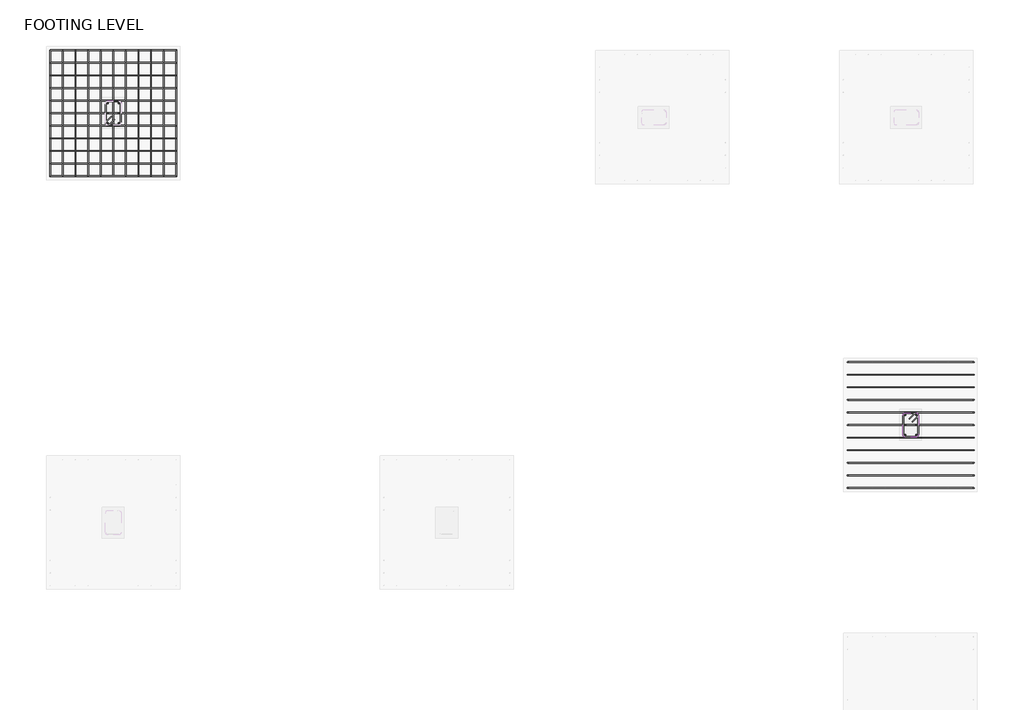
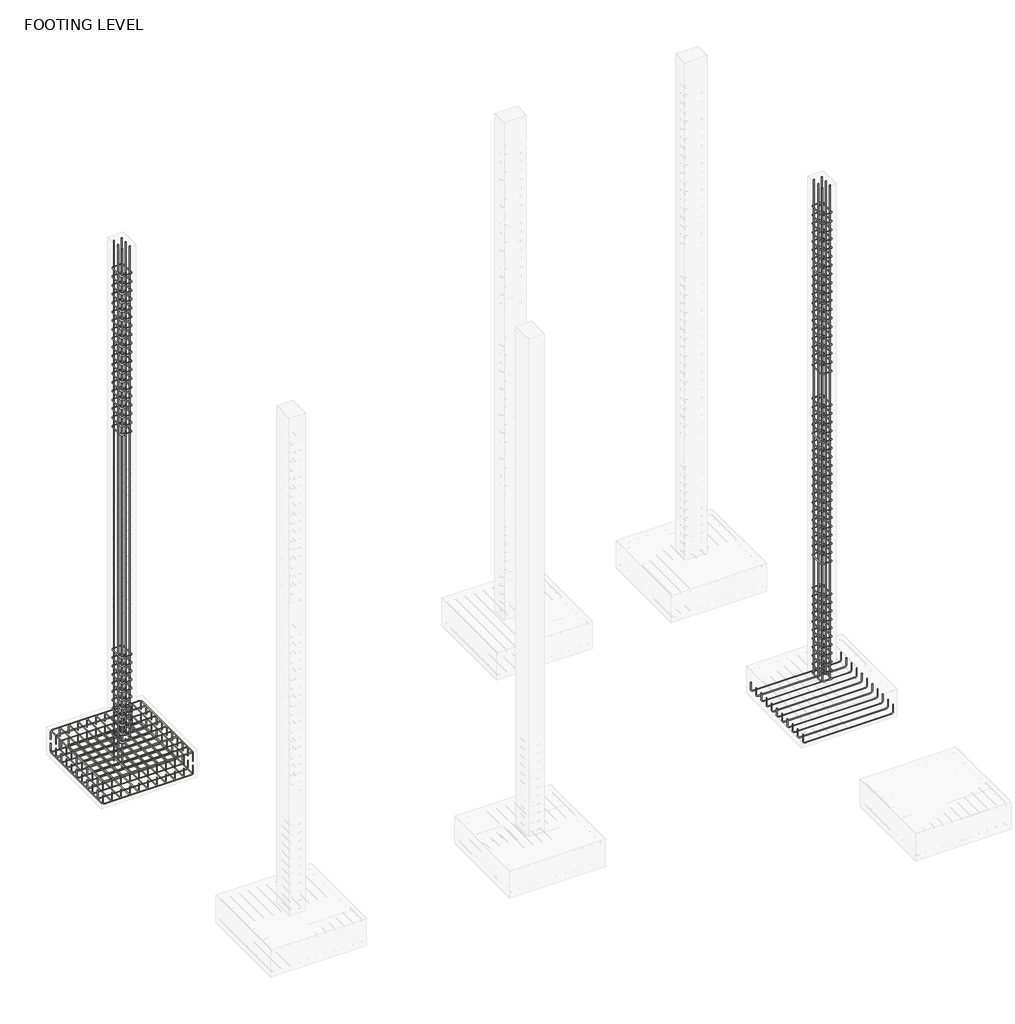
# One storey, part 6 of 9: 22 reinforcing bars.
"""IFC4 building model written with IfcOpenShell, lengths in millimetres."""

from ifc_helpers import new_model, si_unit, point, frame, origin, place, context, project, spatial, polyline, circle_curve, trimmed, segment, composite_curve, source, transform, mapped, element, save
from ifc_brep_helpers import swept_disk

model = new_model("IFC4")

# Units and contexts
model_context = context("Model", 3, world=origin())
ifc_project = project(units=[si_unit("LENGTHUNIT", "METRE", prefix="MILLI")], contexts=[model_context])

# Site, building, storey
site = spatial("IfcSite", under=ifc_project)
building = spatial("IfcBuilding", under=site)
storey = spatial("IfcBuildingStorey", under=building, Name="FOOTING LEVEL", Elevation=-1981.2)

# Reinforcing bars
placement = place(None, origin())
reinforcing_bar_shape = source(origin(), model_context, "Body", "SolidModel", [
    swept_disk(composite_curve([segment(polyline([(-12382.3821491, 8189.9555175, -1938.3375), (-12439.2463461, 8133.0913204, -1938.3375)]), True, "CONTINUOUS"), segment(trimmed(circle_curve(frame((-12422.4083659, 8116.2533402, -1938.3375), z_axis=(0.0, 0.0, 1.0), x_axis=(-16.837980199999947, 16.837980199999947, 0.0)), 23.8125), [point((-12439.2463461, 8133.0913204, -1938.3375))], [point((-12422.4083659, 8092.4408402, -1938.3375))], True, "CARTESIAN"), True, "CONTINUOUS"), segment(polyline([(-12422.4083659, 8092.4408402, -1938.3375), (-12301.7583659, 8092.4408402, -1938.3375)]), True, "CONTINUOUS"), segment(trimmed(circle_curve(frame((-12301.7583659, 8116.2533402, -1938.3375), z_axis=(0.0, 0.0, 1.0), x_axis=(0.0, -23.8125, 0.0)), 23.8125), [point((-12301.7583659, 8092.4408402, -1938.3375))], [point((-12277.9458659, 8116.2533402, -1938.3375))], True, "CARTESIAN"), True, "CONTINUOUS"), segment(polyline([(-12277.9458659, 8116.2533402, -1938.3375), (-12277.9458659, 8338.5033402, -1938.3375)]), True, "CONTINUOUS"), segment(trimmed(circle_curve(frame((-12301.7203098, 8338.5033402, -1939.6832232), z_axis=(-0.056513312022656255, 0.0, 0.9984018457335854), x_axis=(23.774443900001643, 0.0, 1.3457231999998385)), 23.8125), [point((-12277.9458659, 8338.5033402, -1938.3375))], [point((-12301.7203098, 8362.3158402, -1939.6832232))], True, "CARTESIAN"), True, "CONTINUOUS"), segment(polyline([(-12301.7203098, 8362.3158402, -1939.6832232), (-12422.4464219, 8362.3158402, -1946.5167768)]), True, "CONTINUOUS"), segment(trimmed(circle_curve(frame((-12422.4464219, 8338.5033402, -1946.5167768), z_axis=(-0.056513312022656255, 0.0, 0.9984018457335854), x_axis=(0.0, 23.8125, 0.0)), 23.8125), [point((-12422.4464219, 8362.3158402, -1946.5167768))], [point((-12446.2208659, 8338.5033402, -1947.8625))], True, "CARTESIAN"), True, "CONTINUOUS"), segment(polyline([(-12446.2208659, 8338.5033402, -1947.8625), (-12446.2208659, 8116.2533402, -1947.8625)]), True, "CONTINUOUS"), segment(trimmed(circle_curve(frame((-12422.4083659, 8116.2533402, -1947.8625), z_axis=(0.0, 0.0, 1.0), x_axis=(-23.8125, 0.0, 0.0)), 23.8125), [point((-12446.2208659, 8116.2533402, -1947.8625))], [point((-12405.5703857, 8099.41536, -1947.8625))], True, "CARTESIAN"), True, "CONTINUOUS"), segment(polyline([(-12405.5703857, 8099.41536, -1947.8625), (-12348.7061886, 8156.279557, -1947.8625)]), True, "CONTINUOUS")], self_intersect=False), 4.7625),
])
element("IfcReinforcingBar", 1, at=placement, inside=storey, context=model_context, shape_type="MappedRepresentation", body=[
    mapped(reinforcing_bar_shape, transform((0.0, 0.0, 0.0), x_axis=(1.0, 0.0, 0.0), y_axis=(0.0, 1.0, 0.0), z_axis=(0.0, 0.0, 1.0))),
    mapped(reinforcing_bar_shape, transform((0.0, 0.0, 142.5866456), x_axis=(1.0, 0.0, 0.0), y_axis=(0.0, 1.0, 0.0), z_axis=(0.0, 0.0, 1.0))),
    mapped(reinforcing_bar_shape, transform((0.0, 0.0, 285.1732912), x_axis=(1.0, 0.0, 0.0), y_axis=(0.0, 1.0, 0.0), z_axis=(0.0, 0.0, 1.0))),
    mapped(reinforcing_bar_shape, transform((0.0, 0.0, 427.7599369), x_axis=(1.0, 0.0, 0.0), y_axis=(0.0, 1.0, 0.0), z_axis=(0.0, 0.0, 1.0))),
    mapped(reinforcing_bar_shape, transform((0.0, 0.0, 570.3465825), x_axis=(1.0, 0.0, 0.0), y_axis=(0.0, 1.0, 0.0), z_axis=(0.0, 0.0, 1.0))),
    mapped(reinforcing_bar_shape, transform((0.0, 0.0, 712.9332281), x_axis=(1.0, 0.0, 0.0), y_axis=(0.0, 1.0, 0.0), z_axis=(0.0, 0.0, 1.0))),
    mapped(reinforcing_bar_shape, transform((0.0, 0.0, 855.5198737), x_axis=(1.0, 0.0, 0.0), y_axis=(0.0, 1.0, 0.0), z_axis=(0.0, 0.0, 1.0))),
    mapped(reinforcing_bar_shape, transform((0.0, 0.0, 998.1065193), x_axis=(1.0, 0.0, 0.0), y_axis=(0.0, 1.0, 0.0), z_axis=(0.0, 0.0, 1.0))),
    mapped(reinforcing_bar_shape, transform((0.0, 0.0, 1140.6931649), x_axis=(1.0, 0.0, 0.0), y_axis=(0.0, 1.0, 0.0), z_axis=(0.0, 0.0, 1.0))),
    mapped(reinforcing_bar_shape, transform((0.0, 0.0, 1283.2798106), x_axis=(1.0, 0.0, 0.0), y_axis=(0.0, 1.0, 0.0), z_axis=(0.0, 0.0, 1.0))),
    mapped(reinforcing_bar_shape, transform((0.0, 0.0, 1425.8664562), x_axis=(1.0, 0.0, 0.0), y_axis=(0.0, 1.0, 0.0), z_axis=(0.0, 0.0, 1.0))),
])
element("IfcReinforcingBar", 2, at=placement, inside=storey, context=model_context, shape_type="SolidModel", body=[
    swept_disk(composite_curve([segment(polyline([(-12423.8882737, 8340.8596793, -2400.3), (-12423.8882737, 8340.8596793, 6362.7)]), True, "CONTINUOUS")], self_intersect=False), 6.35),
])
element("IfcReinforcingBar", 3, at=placement, inside=storey, context=model_context, shape_type="SolidModel", body=[
    swept_disk(composite_curve([segment(polyline([(-12300.2784581, 8340.8596793, -1943.1), (-12300.2784581, 8340.8596793, 6362.7)]), True, "CONTINUOUS")], self_intersect=False), 6.35),
])
element("IfcReinforcingBar", 4, at=placement, inside=storey, context=model_context, shape_type="SolidModel", body=[
    swept_disk(composite_curve([segment(polyline([(-12423.8882737, 8113.8970011, -2400.3), (-12423.8882737, 8113.8970011, 6362.7)]), True, "CONTINUOUS")], self_intersect=False), 6.35),
])
element("IfcReinforcingBar", 5, at=placement, inside=storey, context=model_context, shape_type="SolidModel", body=[
    swept_disk(composite_curve([segment(polyline([(-12300.2784581, 8113.8970011, -1943.1), (-12300.2784581, 8113.8970011, 6362.7)]), True, "CONTINUOUS")], self_intersect=False), 6.35),
])
element("IfcReinforcingBar", 6, at=placement, inside=storey, context=model_context, shape_type="SolidModel", body=[
    swept_disk(composite_curve([segment(polyline([(-12423.8882737, 8228.1970011, -2400.3), (-12423.8882737, 8228.1970011, 6362.7)]), True, "CONTINUOUS")], self_intersect=False), 6.35),
])
element("IfcReinforcingBar", 7, at=placement, inside=storey, context=model_context, shape_type="SolidModel", body=[
    swept_disk(composite_curve([segment(polyline([(-12300.2784581, 8228.1970011, -1943.1), (-12300.2784581, 8228.1970011, 6362.7)]), True, "CONTINUOUS")], self_intersect=False), 6.35),
])
reinforcing_bar_2_shape = source(origin(), model_context, "Body", "SolidModel", [
    swept_disk(composite_curve([segment(polyline([(-3975.4566189, 3944.9119441, -2247.9), (-3975.4566189, 3944.9119441, -2362.2)]), True, "CONTINUOUS"), segment(trimmed(circle_curve(frame((-3942.1191189, 3944.9119441, -2362.2), z_axis=(0.0, -1.0, 0.0), x_axis=(-33.33750000000009, 0.0, 0.0)), 33.3375), [point((-3975.4566189, 3944.9119441, -2362.2))], [point((-3942.1191189, 3944.9119441, -2395.5375))], True, "CARTESIAN"), True, "CONTINUOUS"), segment(polyline([(-3942.1191189, 3944.9119441, -2395.5375), (-2570.5191189, 3944.9119441, -2395.5375)]), True, "CONTINUOUS"), segment(trimmed(circle_curve(frame((-2570.5191189, 3944.9119441, -2362.2), z_axis=(0.0, -1.0, 0.0), x_axis=(0.0, 0.0, -33.33750000000009)), 33.3375), [point((-2570.5191189, 3944.9119441, -2395.5375))], [point((-2537.1816189, 3944.9119441, -2362.2))], True, "CARTESIAN"), True, "CONTINUOUS"), segment(polyline([(-2537.1816189, 3944.9119441, -2362.2), (-2537.1816189, 3944.9119441, -2247.9)]), True, "CONTINUOUS")], self_intersect=False), 4.7625),
])
element("IfcReinforcingBar", 8, at=placement, inside=storey, context=model_context, shape_type="MappedRepresentation", body=[
    mapped(reinforcing_bar_2_shape, transform((0.0, 0.0, 0.0), x_axis=(1.0, 0.0, 0.0), y_axis=(0.0, 1.0, 0.0), z_axis=(0.0, 0.0, 1.0))),
    mapped(reinforcing_bar_2_shape, transform((0.0, 143.8275, 0.0), x_axis=(1.0, 0.0, 0.0), y_axis=(0.0, 1.0, 0.0), z_axis=(0.0, 0.0, 1.0))),
    mapped(reinforcing_bar_2_shape, transform((0.0, 287.655, 0.0), x_axis=(1.0, 0.0, 0.0), y_axis=(0.0, 1.0, 0.0), z_axis=(0.0, 0.0, 1.0))),
    mapped(reinforcing_bar_2_shape, transform((0.0, 431.4825, 0.0), x_axis=(1.0, 0.0, 0.0), y_axis=(0.0, 1.0, 0.0), z_axis=(0.0, 0.0, 1.0))),
    mapped(reinforcing_bar_2_shape, transform((0.0, 575.31, 0.0), x_axis=(1.0, 0.0, 0.0), y_axis=(0.0, 1.0, 0.0), z_axis=(0.0, 0.0, 1.0))),
    mapped(reinforcing_bar_2_shape, transform((0.0, 719.1375, 0.0), x_axis=(1.0, 0.0, 0.0), y_axis=(0.0, 1.0, 0.0), z_axis=(0.0, 0.0, 1.0))),
    mapped(reinforcing_bar_2_shape, transform((0.0, 862.965, 0.0), x_axis=(1.0, 0.0, 0.0), y_axis=(0.0, 1.0, 0.0), z_axis=(0.0, 0.0, 1.0))),
    mapped(reinforcing_bar_2_shape, transform((0.0, 1006.7925, 0.0), x_axis=(1.0, 0.0, 0.0), y_axis=(0.0, 1.0, 0.0), z_axis=(0.0, 0.0, 1.0))),
    mapped(reinforcing_bar_2_shape, transform((0.0, 1150.62, 0.0), x_axis=(1.0, 0.0, 0.0), y_axis=(0.0, 1.0, 0.0), z_axis=(0.0, 0.0, 1.0))),
    mapped(reinforcing_bar_2_shape, transform((0.0, 1294.4475, 0.0), x_axis=(1.0, 0.0, 0.0), y_axis=(0.0, 1.0, 0.0), z_axis=(0.0, 0.0, 1.0))),
    mapped(reinforcing_bar_2_shape, transform((0.0, 1438.275, 0.0), x_axis=(1.0, 0.0, 0.0), y_axis=(0.0, 1.0, 0.0), z_axis=(0.0, 0.0, 1.0))),
])
reinforcing_bar_3_shape = source(origin(), model_context, "Body", "SolidModel", [
    swept_disk(composite_curve([segment(polyline([(-11642.9458659, 8946.5158402, -2171.7), (-11642.9458659, 8946.5158402, -2057.4)]), True, "CONTINUOUS"), segment(trimmed(circle_curve(frame((-11642.9458659, 8913.1783402, -2057.4), z_axis=(1.0, 0.0, 0.0), x_axis=(0.0, 33.337499999999636, 0.0)), 33.3375), [point((-11642.9458659, 8946.5158402, -2057.4))], [point((-11642.9458659, 8913.1783402, -2024.0625))], True, "CARTESIAN"), True, "CONTINUOUS"), segment(polyline([(-11642.9458659, 8913.1783402, -2024.0625), (-11642.9458659, 7541.5783402, -2024.0625)]), True, "CONTINUOUS"), segment(trimmed(circle_curve(frame((-11642.9458659, 7541.5783402, -2057.4), z_axis=(1.0, 0.0, 0.0), x_axis=(0.0, 0.0, 33.33750000000009)), 33.3375), [point((-11642.9458659, 7541.5783402, -2024.0625))], [point((-11642.9458659, 7508.2408402, -2057.4))], True, "CARTESIAN"), True, "CONTINUOUS"), segment(polyline([(-11642.9458659, 7508.2408402, -2057.4), (-11642.9458659, 7508.2408402, -2171.7)]), True, "CONTINUOUS")], self_intersect=False), 4.7625),
])
element("IfcReinforcingBar", 9, at=placement, inside=storey, context=model_context, shape_type="MappedRepresentation", body=[
    mapped(reinforcing_bar_3_shape, transform((0.0, 0.0, 0.0), x_axis=(1.0, 0.0, 0.0), y_axis=(0.0, 1.0, 0.0), z_axis=(0.0, 0.0, 1.0))),
    mapped(reinforcing_bar_3_shape, transform((-143.8275, 0.0, 0.0), x_axis=(1.0, 0.0, 0.0), y_axis=(0.0, 1.0, 0.0), z_axis=(0.0, 0.0, 1.0))),
    mapped(reinforcing_bar_3_shape, transform((-287.655, 0.0, 0.0), x_axis=(1.0, 0.0, 0.0), y_axis=(0.0, 1.0, 0.0), z_axis=(0.0, 0.0, 1.0))),
    mapped(reinforcing_bar_3_shape, transform((-431.4825, 0.0, 0.0), x_axis=(1.0, 0.0, 0.0), y_axis=(0.0, 1.0, 0.0), z_axis=(0.0, 0.0, 1.0))),
    mapped(reinforcing_bar_3_shape, transform((-575.31, 0.0, 0.0), x_axis=(1.0, 0.0, 0.0), y_axis=(0.0, 1.0, 0.0), z_axis=(0.0, 0.0, 1.0))),
    mapped(reinforcing_bar_3_shape, transform((-719.1375, 0.0, 0.0), x_axis=(1.0, 0.0, 0.0), y_axis=(0.0, 1.0, 0.0), z_axis=(0.0, 0.0, 1.0))),
    mapped(reinforcing_bar_3_shape, transform((-862.965, 0.0, 0.0), x_axis=(1.0, 0.0, 0.0), y_axis=(0.0, 1.0, 0.0), z_axis=(0.0, 0.0, 1.0))),
    mapped(reinforcing_bar_3_shape, transform((-1006.7925, 0.0, 0.0), x_axis=(1.0, 0.0, 0.0), y_axis=(0.0, 1.0, 0.0), z_axis=(0.0, 0.0, 1.0))),
    mapped(reinforcing_bar_3_shape, transform((-1150.62, 0.0, 0.0), x_axis=(1.0, 0.0, 0.0), y_axis=(0.0, 1.0, 0.0), z_axis=(0.0, 0.0, 1.0))),
    mapped(reinforcing_bar_3_shape, transform((-1294.4475, 0.0, 0.0), x_axis=(1.0, 0.0, 0.0), y_axis=(0.0, 1.0, 0.0), z_axis=(0.0, 0.0, 1.0))),
    mapped(reinforcing_bar_3_shape, transform((-1438.275, 0.0, 0.0), x_axis=(1.0, 0.0, 0.0), y_axis=(0.0, 1.0, 0.0), z_axis=(0.0, 0.0, 1.0))),
])
reinforcing_bar_4_shape = source(origin(), model_context, "Body", "SolidModel", [
    swept_disk(composite_curve([segment(polyline([(-11642.9458659, 7508.2408402, -2247.9), (-11642.9458659, 7508.2408402, -2362.2)]), True, "CONTINUOUS"), segment(trimmed(circle_curve(frame((-11642.9458659, 7541.5783402, -2362.2), z_axis=(1.0, 0.0, 0.0), x_axis=(0.0, -33.337499999999636, 0.0)), 33.3375), [point((-11642.9458659, 7508.2408402, -2362.2))], [point((-11642.9458659, 7541.5783402, -2395.5375))], True, "CARTESIAN"), True, "CONTINUOUS"), segment(polyline([(-11642.9458659, 7541.5783402, -2395.5375), (-11642.9458659, 8913.1783402, -2395.5375)]), True, "CONTINUOUS"), segment(trimmed(circle_curve(frame((-11642.9458659, 8913.1783402, -2362.2), z_axis=(1.0, 0.0, 0.0), x_axis=(0.0, 0.0, -33.33750000000009)), 33.3375), [point((-11642.9458659, 8913.1783402, -2395.5375))], [point((-11642.9458659, 8946.5158402, -2362.2))], True, "CARTESIAN"), True, "CONTINUOUS"), segment(polyline([(-11642.9458659, 8946.5158402, -2362.2), (-11642.9458659, 8946.5158402, -2247.9)]), True, "CONTINUOUS")], self_intersect=False), 4.7625),
])
element("IfcReinforcingBar", 10, at=placement, inside=storey, context=model_context, shape_type="MappedRepresentation", body=[
    mapped(reinforcing_bar_4_shape, transform((0.0, 0.0, 0.0), x_axis=(1.0, 0.0, 0.0), y_axis=(0.0, 1.0, 0.0), z_axis=(0.0, 0.0, 1.0))),
    mapped(reinforcing_bar_4_shape, transform((-143.8275, 0.0, 0.0), x_axis=(1.0, 0.0, 0.0), y_axis=(0.0, 1.0, 0.0), z_axis=(0.0, 0.0, 1.0))),
    mapped(reinforcing_bar_4_shape, transform((-287.655, 0.0, 0.0), x_axis=(1.0, 0.0, 0.0), y_axis=(0.0, 1.0, 0.0), z_axis=(0.0, 0.0, 1.0))),
    mapped(reinforcing_bar_4_shape, transform((-431.4825, 0.0, 0.0), x_axis=(1.0, 0.0, 0.0), y_axis=(0.0, 1.0, 0.0), z_axis=(0.0, 0.0, 1.0))),
    mapped(reinforcing_bar_4_shape, transform((-575.31, 0.0, 0.0), x_axis=(1.0, 0.0, 0.0), y_axis=(0.0, 1.0, 0.0), z_axis=(0.0, 0.0, 1.0))),
    mapped(reinforcing_bar_4_shape, transform((-719.1375, 0.0, 0.0), x_axis=(1.0, 0.0, 0.0), y_axis=(0.0, 1.0, 0.0), z_axis=(0.0, 0.0, 1.0))),
    mapped(reinforcing_bar_4_shape, transform((-862.965, 0.0, 0.0), x_axis=(1.0, 0.0, 0.0), y_axis=(0.0, 1.0, 0.0), z_axis=(0.0, 0.0, 1.0))),
    mapped(reinforcing_bar_4_shape, transform((-1006.7925, 0.0, 0.0), x_axis=(1.0, 0.0, 0.0), y_axis=(0.0, 1.0, 0.0), z_axis=(0.0, 0.0, 1.0))),
    mapped(reinforcing_bar_4_shape, transform((-1150.62, 0.0, 0.0), x_axis=(1.0, 0.0, 0.0), y_axis=(0.0, 1.0, 0.0), z_axis=(0.0, 0.0, 1.0))),
    mapped(reinforcing_bar_4_shape, transform((-1294.4475, 0.0, 0.0), x_axis=(1.0, 0.0, 0.0), y_axis=(0.0, 1.0, 0.0), z_axis=(0.0, 0.0, 1.0))),
    mapped(reinforcing_bar_4_shape, transform((-1438.275, 0.0, 0.0), x_axis=(1.0, 0.0, 0.0), y_axis=(0.0, 1.0, 0.0), z_axis=(0.0, 0.0, 1.0))),
])
reinforcing_bar_5_shape = source(origin(), model_context, "Body", "SolidModel", [
    swept_disk(composite_curve([segment(polyline([(-13081.2208659, 8946.5158402, -2171.7), (-13081.2208659, 8946.5158402, -2057.4)]), True, "CONTINUOUS"), segment(trimmed(circle_curve(frame((-13047.8833659, 8946.5158402, -2057.4), z_axis=(0.0, 1.0, 0.0), x_axis=(-33.337500000001455, 0.0, 0.0)), 33.3375), [point((-13081.2208659, 8946.5158402, -2057.4))], [point((-13047.8833659, 8946.5158402, -2024.0625))], True, "CARTESIAN"), True, "CONTINUOUS"), segment(polyline([(-13047.8833659, 8946.5158402, -2024.0625), (-11676.2833659, 8946.5158402, -2024.0625)]), True, "CONTINUOUS"), segment(trimmed(circle_curve(frame((-11676.2833659, 8946.5158402, -2057.4), z_axis=(0.0, 1.0, 0.0), x_axis=(0.0, 0.0, 33.33750000000009)), 33.3375), [point((-11676.2833659, 8946.5158402, -2024.0625))], [point((-11642.9458659, 8946.5158402, -2057.4))], True, "CARTESIAN"), True, "CONTINUOUS"), segment(polyline([(-11642.9458659, 8946.5158402, -2057.4), (-11642.9458659, 8946.5158402, -2171.7)]), True, "CONTINUOUS")], self_intersect=False), 4.7625),
])
element("IfcReinforcingBar", 11, at=placement, inside=storey, context=model_context, shape_type="MappedRepresentation", body=[
    mapped(reinforcing_bar_5_shape, transform((0.0, 0.0, 0.0), x_axis=(1.0, 0.0, 0.0), y_axis=(0.0, 1.0, 0.0), z_axis=(0.0, 0.0, 1.0))),
    mapped(reinforcing_bar_5_shape, transform((0.0, -143.8275, 0.0), x_axis=(1.0, 0.0, 0.0), y_axis=(0.0, 1.0, 0.0), z_axis=(0.0, 0.0, 1.0))),
    mapped(reinforcing_bar_5_shape, transform((0.0, -287.655, 0.0), x_axis=(1.0, 0.0, 0.0), y_axis=(0.0, 1.0, 0.0), z_axis=(0.0, 0.0, 1.0))),
    mapped(reinforcing_bar_5_shape, transform((0.0, -431.4825, 0.0), x_axis=(1.0, 0.0, 0.0), y_axis=(0.0, 1.0, 0.0), z_axis=(0.0, 0.0, 1.0))),
    mapped(reinforcing_bar_5_shape, transform((0.0, -575.31, 0.0), x_axis=(1.0, 0.0, 0.0), y_axis=(0.0, 1.0, 0.0), z_axis=(0.0, 0.0, 1.0))),
    mapped(reinforcing_bar_5_shape, transform((0.0, -719.1375, 0.0), x_axis=(1.0, 0.0, 0.0), y_axis=(0.0, 1.0, 0.0), z_axis=(0.0, 0.0, 1.0))),
    mapped(reinforcing_bar_5_shape, transform((0.0, -862.965, 0.0), x_axis=(1.0, 0.0, 0.0), y_axis=(0.0, 1.0, 0.0), z_axis=(0.0, 0.0, 1.0))),
    mapped(reinforcing_bar_5_shape, transform((0.0, -1006.7925, 0.0), x_axis=(1.0, 0.0, 0.0), y_axis=(0.0, 1.0, 0.0), z_axis=(0.0, 0.0, 1.0))),
    mapped(reinforcing_bar_5_shape, transform((0.0, -1150.62, 0.0), x_axis=(1.0, 0.0, 0.0), y_axis=(0.0, 1.0, 0.0), z_axis=(0.0, 0.0, 1.0))),
    mapped(reinforcing_bar_5_shape, transform((0.0, -1294.4475, 0.0), x_axis=(1.0, 0.0, 0.0), y_axis=(0.0, 1.0, 0.0), z_axis=(0.0, 0.0, 1.0))),
    mapped(reinforcing_bar_5_shape, transform((0.0, -1438.275, 0.0), x_axis=(1.0, 0.0, 0.0), y_axis=(0.0, 1.0, 0.0), z_axis=(0.0, 0.0, 1.0))),
])
reinforcing_bar_6_shape = source(origin(), model_context, "Body", "SolidModel", [
    swept_disk(composite_curve([segment(polyline([(-13081.2208659, 7508.2408402, -2247.9), (-13081.2208659, 7508.2408402, -2362.2)]), True, "CONTINUOUS"), segment(trimmed(circle_curve(frame((-13047.8833659, 7508.2408402, -2362.2), z_axis=(0.0, -1.0, 0.0), x_axis=(-33.337500000001455, 0.0, 0.0)), 33.3375), [point((-13081.2208659, 7508.2408402, -2362.2))], [point((-13047.8833659, 7508.2408402, -2395.5375))], True, "CARTESIAN"), True, "CONTINUOUS"), segment(polyline([(-13047.8833659, 7508.2408402, -2395.5375), (-11676.2833659, 7508.2408402, -2395.5375)]), True, "CONTINUOUS"), segment(trimmed(circle_curve(frame((-11676.2833659, 7508.2408402, -2362.2), z_axis=(0.0, -1.0, 0.0), x_axis=(0.0, 0.0, -33.33750000000009)), 33.3375), [point((-11676.2833659, 7508.2408402, -2395.5375))], [point((-11642.9458659, 7508.2408402, -2362.2))], True, "CARTESIAN"), True, "CONTINUOUS"), segment(polyline([(-11642.9458659, 7508.2408402, -2362.2), (-11642.9458659, 7508.2408402, -2247.9)]), True, "CONTINUOUS")], self_intersect=False), 4.7625),
])
element("IfcReinforcingBar", 12, at=placement, inside=storey, context=model_context, shape_type="MappedRepresentation", body=[
    mapped(reinforcing_bar_6_shape, transform((0.0, 0.0, 0.0), x_axis=(1.0, 0.0, 0.0), y_axis=(0.0, 1.0, 0.0), z_axis=(0.0, 0.0, 1.0))),
    mapped(reinforcing_bar_6_shape, transform((0.0, 143.8275, 0.0), x_axis=(1.0, 0.0, 0.0), y_axis=(0.0, 1.0, 0.0), z_axis=(0.0, 0.0, 1.0))),
    mapped(reinforcing_bar_6_shape, transform((0.0, 287.655, 0.0), x_axis=(1.0, 0.0, 0.0), y_axis=(0.0, 1.0, 0.0), z_axis=(0.0, 0.0, 1.0))),
    mapped(reinforcing_bar_6_shape, transform((0.0, 431.4825, 0.0), x_axis=(1.0, 0.0, 0.0), y_axis=(0.0, 1.0, 0.0), z_axis=(0.0, 0.0, 1.0))),
    mapped(reinforcing_bar_6_shape, transform((0.0, 575.31, 0.0), x_axis=(1.0, 0.0, 0.0), y_axis=(0.0, 1.0, 0.0), z_axis=(0.0, 0.0, 1.0))),
    mapped(reinforcing_bar_6_shape, transform((0.0, 719.1375, 0.0), x_axis=(1.0, 0.0, 0.0), y_axis=(0.0, 1.0, 0.0), z_axis=(0.0, 0.0, 1.0))),
    mapped(reinforcing_bar_6_shape, transform((0.0, 862.965, 0.0), x_axis=(1.0, 0.0, 0.0), y_axis=(0.0, 1.0, 0.0), z_axis=(0.0, 0.0, 1.0))),
    mapped(reinforcing_bar_6_shape, transform((0.0, 1006.7925, 0.0), x_axis=(1.0, 0.0, 0.0), y_axis=(0.0, 1.0, 0.0), z_axis=(0.0, 0.0, 1.0))),
    mapped(reinforcing_bar_6_shape, transform((0.0, 1150.62, 0.0), x_axis=(1.0, 0.0, 0.0), y_axis=(0.0, 1.0, 0.0), z_axis=(0.0, 0.0, 1.0))),
    mapped(reinforcing_bar_6_shape, transform((0.0, 1294.4475, 0.0), x_axis=(1.0, 0.0, 0.0), y_axis=(0.0, 1.0, 0.0), z_axis=(0.0, 0.0, 1.0))),
    mapped(reinforcing_bar_6_shape, transform((0.0, 1438.275, 0.0), x_axis=(1.0, 0.0, 0.0), y_axis=(0.0, 1.0, 0.0), z_axis=(0.0, 0.0, 1.0))),
])
reinforcing_bar_7_shape = source(origin(), model_context, "Body", "SolidModel", [
    swept_disk(composite_curve([segment(polyline([(-3236.0203358, 4701.4722668, -1938.3375), (-3179.1561387, 4758.3364639, -1938.3375)]), True, "CONTINUOUS"), segment(trimmed(circle_curve(frame((-3195.9941189, 4775.1744441, -1938.3375), z_axis=(0.0, 0.0, 1.0), x_axis=(16.837980199999947, -16.837980199999947, 0.0)), 23.8125), [point((-3179.1561387, 4758.3364639, -1938.3375))], [point((-3195.9941189, 4798.9869441, -1938.3375))], True, "CARTESIAN"), True, "CONTINUOUS"), segment(polyline([(-3195.9941189, 4798.9869441, -1938.3375), (-3316.6441189, 4798.9869441, -1938.3375)]), True, "CONTINUOUS"), segment(trimmed(circle_curve(frame((-3316.6441189, 4775.1744441, -1938.3375), z_axis=(0.0, 0.0, 1.0), x_axis=(0.0, 23.8125, 0.0)), 23.8125), [point((-3316.6441189, 4798.9869441, -1938.3375))], [point((-3340.4566189, 4775.1744441, -1938.3375))], True, "CARTESIAN"), True, "CONTINUOUS"), segment(polyline([(-3340.4566189, 4775.1744441, -1938.3375), (-3340.4566189, 4552.9244441, -1938.3375)]), True, "CONTINUOUS"), segment(trimmed(circle_curve(frame((-3316.682175, 4552.9244441, -1939.6832232), z_axis=(0.056513312022656255, 0.0, 0.9984018457335854), x_axis=(-23.77444390000028, 0.0, 1.3457231999998385)), 23.8125), [point((-3340.4566189, 4552.9244441, -1938.3375))], [point((-3316.682175, 4529.1119441, -1939.6832232))], True, "CARTESIAN"), True, "CONTINUOUS"), segment(polyline([(-3316.682175, 4529.1119441, -1939.6832232), (-3195.9560629, 4529.1119441, -1946.5167768)]), True, "CONTINUOUS"), segment(trimmed(circle_curve(frame((-3195.9560629, 4552.9244441, -1946.5167768), z_axis=(0.056513312022656255, 0.0, 0.9984018457335854), x_axis=(0.0, -23.8125, 0.0)), 23.8125), [point((-3195.9560629, 4529.1119441, -1946.5167768))], [point((-3172.1816189, 4552.9244441, -1947.8625))], True, "CARTESIAN"), True, "CONTINUOUS"), segment(polyline([(-3172.1816189, 4552.9244441, -1947.8625), (-3172.1816189, 4775.1744441, -1947.8625)]), True, "CONTINUOUS"), segment(trimmed(circle_curve(frame((-3195.9941189, 4775.1744441, -1947.8625), z_axis=(0.0, 0.0, 1.0), x_axis=(23.8125, 0.0, 0.0)), 23.8125), [point((-3172.1816189, 4775.1744441, -1947.8625))], [point((-3212.8320991, 4792.0124243, -1947.8625))], True, "CARTESIAN"), True, "CONTINUOUS"), segment(polyline([(-3212.8320991, 4792.0124243, -1947.8625), (-3269.6962962, 4735.1482272, -1947.8625)]), True, "CONTINUOUS")], self_intersect=False), 4.7625),
])
element("IfcReinforcingBar", 13, at=placement, inside=storey, context=model_context, shape_type="MappedRepresentation", body=[
    mapped(reinforcing_bar_7_shape, transform((0.0, 0.0, 0.0), x_axis=(1.0, 0.0, 0.0), y_axis=(0.0, 1.0, 0.0), z_axis=(0.0, 0.0, 1.0))),
    mapped(reinforcing_bar_7_shape, transform((0.0, 0.0, 142.5866456), x_axis=(1.0, 0.0, 0.0), y_axis=(0.0, 1.0, 0.0), z_axis=(0.0, 0.0, 1.0))),
    mapped(reinforcing_bar_7_shape, transform((0.0, 0.0, 285.1732912), x_axis=(1.0, 0.0, 0.0), y_axis=(0.0, 1.0, 0.0), z_axis=(0.0, 0.0, 1.0))),
    mapped(reinforcing_bar_7_shape, transform((0.0, 0.0, 427.7599369), x_axis=(1.0, 0.0, 0.0), y_axis=(0.0, 1.0, 0.0), z_axis=(0.0, 0.0, 1.0))),
    mapped(reinforcing_bar_7_shape, transform((0.0, 0.0, 570.3465825), x_axis=(1.0, 0.0, 0.0), y_axis=(0.0, 1.0, 0.0), z_axis=(0.0, 0.0, 1.0))),
    mapped(reinforcing_bar_7_shape, transform((0.0, 0.0, 712.9332281), x_axis=(1.0, 0.0, 0.0), y_axis=(0.0, 1.0, 0.0), z_axis=(0.0, 0.0, 1.0))),
    mapped(reinforcing_bar_7_shape, transform((0.0, 0.0, 855.5198737), x_axis=(1.0, 0.0, 0.0), y_axis=(0.0, 1.0, 0.0), z_axis=(0.0, 0.0, 1.0))),
    mapped(reinforcing_bar_7_shape, transform((0.0, 0.0, 998.1065193), x_axis=(1.0, 0.0, 0.0), y_axis=(0.0, 1.0, 0.0), z_axis=(0.0, 0.0, 1.0))),
    mapped(reinforcing_bar_7_shape, transform((0.0, 0.0, 1140.6931649), x_axis=(1.0, 0.0, 0.0), y_axis=(0.0, 1.0, 0.0), z_axis=(0.0, 0.0, 1.0))),
    mapped(reinforcing_bar_7_shape, transform((0.0, 0.0, 1283.2798106), x_axis=(1.0, 0.0, 0.0), y_axis=(0.0, 1.0, 0.0), z_axis=(0.0, 0.0, 1.0))),
    mapped(reinforcing_bar_7_shape, transform((0.0, 0.0, 1425.8664562), x_axis=(1.0, 0.0, 0.0), y_axis=(0.0, 1.0, 0.0), z_axis=(0.0, 0.0, 1.0))),
])
element("IfcReinforcingBar", 14, at=placement, inside=storey, context=model_context, shape_type="SolidModel", body=[
    swept_disk(composite_curve([segment(polyline([(-3194.5142111, 4550.568105, -1943.1), (-3194.5142111, 4550.568105, 6362.7)]), True, "CONTINUOUS")], self_intersect=False), 6.35),
])
element("IfcReinforcingBar", 15, at=placement, inside=storey, context=model_context, shape_type="SolidModel", body=[
    swept_disk(composite_curve([segment(polyline([(-3318.1240267, 4550.568105, -1943.1), (-3318.1240267, 4550.568105, 6362.7)]), True, "CONTINUOUS")], self_intersect=False), 6.35),
])
element("IfcReinforcingBar", 16, at=placement, inside=storey, context=model_context, shape_type="SolidModel", body=[
    swept_disk(composite_curve([segment(polyline([(-3194.5142111, 4777.5307832, -1943.1), (-3194.5142111, 4777.5307832, 6362.7)]), True, "CONTINUOUS")], self_intersect=False), 6.35),
])
element("IfcReinforcingBar", 17, at=placement, inside=storey, context=model_context, shape_type="SolidModel", body=[
    swept_disk(composite_curve([segment(polyline([(-3318.1240267, 4777.5307832, -1943.1), (-3318.1240267, 4777.5307832, 6362.7)]), True, "CONTINUOUS")], self_intersect=False), 6.35),
])
element("IfcReinforcingBar", 18, at=placement, inside=storey, context=model_context, shape_type="SolidModel", body=[
    swept_disk(composite_curve([segment(polyline([(-3194.5142111, 4663.2307832, -1943.1), (-3194.5142111, 4663.2307832, 6362.7)]), True, "CONTINUOUS")], self_intersect=False), 6.35),
])
element("IfcReinforcingBar", 19, at=placement, inside=storey, context=model_context, shape_type="SolidModel", body=[
    swept_disk(composite_curve([segment(polyline([(-3318.1240267, 4663.2307832, -1943.1), (-3318.1240267, 4663.2307832, 6362.7)]), True, "CONTINUOUS")], self_intersect=False), 6.35),
])
reinforcing_bar_8_shape = source(origin(), model_context, "Body", "SolidModel", [
    swept_disk(composite_curve([segment(polyline([(-12382.3821491, 8189.9555175, 3243.2625), (-12439.2463461, 8133.0913204, 3243.2625)]), True, "CONTINUOUS"), segment(trimmed(circle_curve(frame((-12422.4083659, 8116.2533402, 3243.2625), z_axis=(0.0, 0.0, 1.0), x_axis=(-16.837980199999947, 16.837980199999947, 0.0)), 23.8125), [point((-12439.2463461, 8133.0913204, 3243.2625))], [point((-12422.4083659, 8092.4408402, 3243.2625))], True, "CARTESIAN"), True, "CONTINUOUS"), segment(polyline([(-12422.4083659, 8092.4408402, 3243.2625), (-12301.7583659, 8092.4408402, 3243.2625)]), True, "CONTINUOUS"), segment(trimmed(circle_curve(frame((-12301.7583659, 8116.2533402, 3243.2625), z_axis=(0.0, 0.0, 1.0), x_axis=(0.0, -23.8125, 0.0)), 23.8125), [point((-12301.7583659, 8092.4408402, 3243.2625))], [point((-12277.9458659, 8116.2533402, 3243.2625))], True, "CARTESIAN"), True, "CONTINUOUS"), segment(polyline([(-12277.9458659, 8116.2533402, 3243.2625), (-12277.9458659, 8338.5033402, 3243.2625)]), True, "CONTINUOUS"), segment(trimmed(circle_curve(frame((-12301.7203098, 8338.5033402, 3241.9167768), z_axis=(-0.056513312022656255, 0.0, 0.9984018457335854), x_axis=(23.774443900001643, 0.0, 1.345723199999611)), 23.8125), [point((-12277.9458659, 8338.5033402, 3243.2625))], [point((-12301.7203098, 8362.3158402, 3241.9167768))], True, "CARTESIAN"), True, "CONTINUOUS"), segment(polyline([(-12301.7203098, 8362.3158402, 3241.9167768), (-12422.4464219, 8362.3158402, 3235.0832232)]), True, "CONTINUOUS"), segment(trimmed(circle_curve(frame((-12422.4464219, 8338.5033402, 3235.0832232), z_axis=(-0.056513312022656255, 0.0, 0.9984018457335854), x_axis=(0.0, 23.8125, 0.0)), 23.8125), [point((-12422.4464219, 8362.3158402, 3235.0832232))], [point((-12446.2208659, 8338.5033402, 3233.7375))], True, "CARTESIAN"), True, "CONTINUOUS"), segment(polyline([(-12446.2208659, 8338.5033402, 3233.7375), (-12446.2208659, 8116.2533402, 3233.7375)]), True, "CONTINUOUS"), segment(trimmed(circle_curve(frame((-12422.4083659, 8116.2533402, 3233.7375), z_axis=(0.0, 0.0, 1.0), x_axis=(-23.8125, 0.0, 0.0)), 23.8125), [point((-12446.2208659, 8116.2533402, 3233.7375))], [point((-12405.5703857, 8099.41536, 3233.7375))], True, "CARTESIAN"), True, "CONTINUOUS"), segment(polyline([(-12405.5703857, 8099.41536, 3233.7375), (-12348.7061886, 8156.279557, 3233.7375)]), True, "CONTINUOUS")], self_intersect=False), 4.7625),
])
element("IfcReinforcingBar", 20, at=placement, inside=storey, context=model_context, shape_type="MappedRepresentation", body=[
    mapped(reinforcing_bar_8_shape, transform((0.0, 0.0, 0.0), x_axis=(1.0, 0.0, 0.0), y_axis=(0.0, 1.0, 0.0), z_axis=(0.0, 0.0, 1.0))),
    mapped(reinforcing_bar_8_shape, transform((0.0, 0.0, 148.4372585), x_axis=(1.0, 0.0, 0.0), y_axis=(0.0, 1.0, 0.0), z_axis=(0.0, 0.0, 1.0))),
    mapped(reinforcing_bar_8_shape, transform((0.0, 0.0, 296.8745169), x_axis=(1.0, 0.0, 0.0), y_axis=(0.0, 1.0, 0.0), z_axis=(0.0, 0.0, 1.0))),
    mapped(reinforcing_bar_8_shape, transform((0.0, 0.0, 445.3117754), x_axis=(1.0, 0.0, 0.0), y_axis=(0.0, 1.0, 0.0), z_axis=(0.0, 0.0, 1.0))),
    mapped(reinforcing_bar_8_shape, transform((0.0, 0.0, 593.7490338), x_axis=(1.0, 0.0, 0.0), y_axis=(0.0, 1.0, 0.0), z_axis=(0.0, 0.0, 1.0))),
    mapped(reinforcing_bar_8_shape, transform((0.0, 0.0, 742.1862923), x_axis=(1.0, 0.0, 0.0), y_axis=(0.0, 1.0, 0.0), z_axis=(0.0, 0.0, 1.0))),
    mapped(reinforcing_bar_8_shape, transform((0.0, 0.0, 890.6235507), x_axis=(1.0, 0.0, 0.0), y_axis=(0.0, 1.0, 0.0), z_axis=(0.0, 0.0, 1.0))),
    mapped(reinforcing_bar_8_shape, transform((0.0, 0.0, 1039.0608092), x_axis=(1.0, 0.0, 0.0), y_axis=(0.0, 1.0, 0.0), z_axis=(0.0, 0.0, 1.0))),
    mapped(reinforcing_bar_8_shape, transform((0.0, 0.0, 1187.4980677), x_axis=(1.0, 0.0, 0.0), y_axis=(0.0, 1.0, 0.0), z_axis=(0.0, 0.0, 1.0))),
    mapped(reinforcing_bar_8_shape, transform((0.0, 0.0, 1335.9353261), x_axis=(1.0, 0.0, 0.0), y_axis=(0.0, 1.0, 0.0), z_axis=(0.0, 0.0, 1.0))),
    mapped(reinforcing_bar_8_shape, transform((0.0, 0.0, 1484.3725846), x_axis=(1.0, 0.0, 0.0), y_axis=(0.0, 1.0, 0.0), z_axis=(0.0, 0.0, 1.0))),
    mapped(reinforcing_bar_8_shape, transform((0.0, 0.0, 1632.809843), x_axis=(1.0, 0.0, 0.0), y_axis=(0.0, 1.0, 0.0), z_axis=(0.0, 0.0, 1.0))),
    mapped(reinforcing_bar_8_shape, transform((0.0, 0.0, 1781.2471015), x_axis=(1.0, 0.0, 0.0), y_axis=(0.0, 1.0, 0.0), z_axis=(0.0, 0.0, 1.0))),
    mapped(reinforcing_bar_8_shape, transform((0.0, 0.0, 1929.6843599), x_axis=(1.0, 0.0, 0.0), y_axis=(0.0, 1.0, 0.0), z_axis=(0.0, 0.0, 1.0))),
    mapped(reinforcing_bar_8_shape, transform((0.0, 0.0, 2078.1216184), x_axis=(1.0, 0.0, 0.0), y_axis=(0.0, 1.0, 0.0), z_axis=(0.0, 0.0, 1.0))),
    mapped(reinforcing_bar_8_shape, transform((0.0, 0.0, 2226.5588768), x_axis=(1.0, 0.0, 0.0), y_axis=(0.0, 1.0, 0.0), z_axis=(0.0, 0.0, 1.0))),
    mapped(reinforcing_bar_8_shape, transform((0.0, 0.0, 2374.9961353), x_axis=(1.0, 0.0, 0.0), y_axis=(0.0, 1.0, 0.0), z_axis=(0.0, 0.0, 1.0))),
    mapped(reinforcing_bar_8_shape, transform((0.0, 0.0, 2523.4333938), x_axis=(1.0, 0.0, 0.0), y_axis=(0.0, 1.0, 0.0), z_axis=(0.0, 0.0, 1.0))),
    mapped(reinforcing_bar_8_shape, transform((0.0, 0.0, 2671.8706522), x_axis=(1.0, 0.0, 0.0), y_axis=(0.0, 1.0, 0.0), z_axis=(0.0, 0.0, 1.0))),
])
reinforcing_bar_9_shape = source(origin(), model_context, "Body", "SolidModel", [
    swept_disk(composite_curve([segment(polyline([(-3236.0203358, 4701.4722668, 42.8625), (-3179.1561387, 4758.3364639, 42.8625)]), True, "CONTINUOUS"), segment(trimmed(circle_curve(frame((-3195.9941189, 4775.1744441, 42.8625), z_axis=(0.0, 0.0, 1.0), x_axis=(16.837980199999947, -16.837980199999947, 0.0)), 23.8125), [point((-3179.1561387, 4758.3364639, 42.8625))], [point((-3195.9941189, 4798.9869441, 42.8625))], True, "CARTESIAN"), True, "CONTINUOUS"), segment(polyline([(-3195.9941189, 4798.9869441, 42.8625), (-3316.6441189, 4798.9869441, 42.8625)]), True, "CONTINUOUS"), segment(trimmed(circle_curve(frame((-3316.6441189, 4775.1744441, 42.8625), z_axis=(0.0, 0.0, 1.0), x_axis=(0.0, 23.8125, 0.0)), 23.8125), [point((-3316.6441189, 4798.9869441, 42.8625))], [point((-3340.4566189, 4775.1744441, 42.8625))], True, "CARTESIAN"), True, "CONTINUOUS"), segment(polyline([(-3340.4566189, 4775.1744441, 42.8625), (-3340.4566189, 4552.9244441, 42.8625)]), True, "CONTINUOUS"), segment(trimmed(circle_curve(frame((-3316.682175, 4552.9244441, 41.5167768), z_axis=(0.056513312022656255, 0.0, 0.9984018457335854), x_axis=(-23.77444390000028, 0.0, 1.3457231999999948)), 23.8125), [point((-3340.4566189, 4552.9244441, 42.8625))], [point((-3316.682175, 4529.1119441, 41.5167768))], True, "CARTESIAN"), True, "CONTINUOUS"), segment(polyline([(-3316.682175, 4529.1119441, 41.5167768), (-3195.9560629, 4529.1119441, 34.6832232)]), True, "CONTINUOUS"), segment(trimmed(circle_curve(frame((-3195.9560629, 4552.9244441, 34.6832232), z_axis=(0.056513312022656255, 0.0, 0.9984018457335854), x_axis=(0.0, -23.8125, 0.0)), 23.8125), [point((-3195.9560629, 4529.1119441, 34.6832232))], [point((-3172.1816189, 4552.9244441, 33.3375))], True, "CARTESIAN"), True, "CONTINUOUS"), segment(polyline([(-3172.1816189, 4552.9244441, 33.3375), (-3172.1816189, 4775.1744441, 33.3375)]), True, "CONTINUOUS"), segment(trimmed(circle_curve(frame((-3195.9941189, 4775.1744441, 33.3375), z_axis=(0.0, 0.0, 1.0), x_axis=(23.8125, 0.0, 0.0)), 23.8125), [point((-3172.1816189, 4775.1744441, 33.3375))], [point((-3212.8320991, 4792.0124243, 33.3375))], True, "CARTESIAN"), True, "CONTINUOUS"), segment(polyline([(-3212.8320991, 4792.0124243, 33.3375), (-3269.6962962, 4735.1482272, 33.3375)]), True, "CONTINUOUS")], self_intersect=False), 4.7625),
])
element("IfcReinforcingBar", 21, at=placement, inside=storey, context=model_context, shape_type="MappedRepresentation", body=[
    mapped(reinforcing_bar_9_shape, transform((0.0, 0.0, 0.0), x_axis=(1.0, 0.0, 0.0), y_axis=(0.0, 1.0, 0.0), z_axis=(0.0, 0.0, 1.0))),
    mapped(reinforcing_bar_9_shape, transform((0.0, 0.0, 146.2204368), x_axis=(1.0, 0.0, 0.0), y_axis=(0.0, 1.0, 0.0), z_axis=(0.0, 0.0, 1.0))),
    mapped(reinforcing_bar_9_shape, transform((0.0, 0.0, 292.4408736), x_axis=(1.0, 0.0, 0.0), y_axis=(0.0, 1.0, 0.0), z_axis=(0.0, 0.0, 1.0))),
    mapped(reinforcing_bar_9_shape, transform((0.0, 0.0, 438.6613104), x_axis=(1.0, 0.0, 0.0), y_axis=(0.0, 1.0, 0.0), z_axis=(0.0, 0.0, 1.0))),
    mapped(reinforcing_bar_9_shape, transform((0.0, 0.0, 584.8817472), x_axis=(1.0, 0.0, 0.0), y_axis=(0.0, 1.0, 0.0), z_axis=(0.0, 0.0, 1.0))),
    mapped(reinforcing_bar_9_shape, transform((0.0, 0.0, 731.102184), x_axis=(1.0, 0.0, 0.0), y_axis=(0.0, 1.0, 0.0), z_axis=(0.0, 0.0, 1.0))),
    mapped(reinforcing_bar_9_shape, transform((0.0, 0.0, 877.3226208), x_axis=(1.0, 0.0, 0.0), y_axis=(0.0, 1.0, 0.0), z_axis=(0.0, 0.0, 1.0))),
    mapped(reinforcing_bar_9_shape, transform((0.0, 0.0, 1023.5430576), x_axis=(1.0, 0.0, 0.0), y_axis=(0.0, 1.0, 0.0), z_axis=(0.0, 0.0, 1.0))),
    mapped(reinforcing_bar_9_shape, transform((0.0, 0.0, 1169.7634944), x_axis=(1.0, 0.0, 0.0), y_axis=(0.0, 1.0, 0.0), z_axis=(0.0, 0.0, 1.0))),
    mapped(reinforcing_bar_9_shape, transform((0.0, 0.0, 1315.9839312), x_axis=(1.0, 0.0, 0.0), y_axis=(0.0, 1.0, 0.0), z_axis=(0.0, 0.0, 1.0))),
    mapped(reinforcing_bar_9_shape, transform((0.0, 0.0, 1462.2043681), x_axis=(1.0, 0.0, 0.0), y_axis=(0.0, 1.0, 0.0), z_axis=(0.0, 0.0, 1.0))),
    mapped(reinforcing_bar_9_shape, transform((0.0, 0.0, 1608.4248049), x_axis=(1.0, 0.0, 0.0), y_axis=(0.0, 1.0, 0.0), z_axis=(0.0, 0.0, 1.0))),
    mapped(reinforcing_bar_9_shape, transform((0.0, 0.0, 1754.6452417), x_axis=(1.0, 0.0, 0.0), y_axis=(0.0, 1.0, 0.0), z_axis=(0.0, 0.0, 1.0))),
    mapped(reinforcing_bar_9_shape, transform((0.0, 0.0, 1900.8656785), x_axis=(1.0, 0.0, 0.0), y_axis=(0.0, 1.0, 0.0), z_axis=(0.0, 0.0, 1.0))),
    mapped(reinforcing_bar_9_shape, transform((0.0, 0.0, 2047.0861153), x_axis=(1.0, 0.0, 0.0), y_axis=(0.0, 1.0, 0.0), z_axis=(0.0, 0.0, 1.0))),
    mapped(reinforcing_bar_9_shape, transform((0.0, 0.0, 2193.3065521), x_axis=(1.0, 0.0, 0.0), y_axis=(0.0, 1.0, 0.0), z_axis=(0.0, 0.0, 1.0))),
    mapped(reinforcing_bar_9_shape, transform((0.0, 0.0, 2339.5269889), x_axis=(1.0, 0.0, 0.0), y_axis=(0.0, 1.0, 0.0), z_axis=(0.0, 0.0, 1.0))),
    mapped(reinforcing_bar_9_shape, transform((0.0, 0.0, 2485.7474257), x_axis=(1.0, 0.0, 0.0), y_axis=(0.0, 1.0, 0.0), z_axis=(0.0, 0.0, 1.0))),
    mapped(reinforcing_bar_9_shape, transform((0.0, 0.0, 2631.9678625), x_axis=(1.0, 0.0, 0.0), y_axis=(0.0, 1.0, 0.0), z_axis=(0.0, 0.0, 1.0))),
])
reinforcing_bar_10_shape = source(origin(), model_context, "Body", "SolidModel", [
    swept_disk(composite_curve([segment(polyline([(-3236.0203358, 4701.4722668, 3243.2625), (-3179.1561387, 4758.3364639, 3243.2625)]), True, "CONTINUOUS"), segment(trimmed(circle_curve(frame((-3195.9941189, 4775.1744441, 3243.2625), z_axis=(0.0, 0.0, 1.0), x_axis=(16.837980199999947, -16.837980199999947, 0.0)), 23.8125), [point((-3179.1561387, 4758.3364639, 3243.2625))], [point((-3195.9941189, 4798.9869441, 3243.2625))], True, "CARTESIAN"), True, "CONTINUOUS"), segment(polyline([(-3195.9941189, 4798.9869441, 3243.2625), (-3316.6441189, 4798.9869441, 3243.2625)]), True, "CONTINUOUS"), segment(trimmed(circle_curve(frame((-3316.6441189, 4775.1744441, 3243.2625), z_axis=(0.0, 0.0, 1.0), x_axis=(0.0, 23.8125, 0.0)), 23.8125), [point((-3316.6441189, 4798.9869441, 3243.2625))], [point((-3340.4566189, 4775.1744441, 3243.2625))], True, "CARTESIAN"), True, "CONTINUOUS"), segment(polyline([(-3340.4566189, 4775.1744441, 3243.2625), (-3340.4566189, 4552.9244441, 3243.2625)]), True, "CONTINUOUS"), segment(trimmed(circle_curve(frame((-3316.682175, 4552.9244441, 3241.9167768), z_axis=(0.056513312022656255, 0.0, 0.9984018457335854), x_axis=(-23.77444390000028, 0.0, 1.345723199999611)), 23.8125), [point((-3340.4566189, 4552.9244441, 3243.2625))], [point((-3316.682175, 4529.1119441, 3241.9167768))], True, "CARTESIAN"), True, "CONTINUOUS"), segment(polyline([(-3316.682175, 4529.1119441, 3241.9167768), (-3195.9560629, 4529.1119441, 3235.0832232)]), True, "CONTINUOUS"), segment(trimmed(circle_curve(frame((-3195.9560629, 4552.9244441, 3235.0832232), z_axis=(0.056513312022656255, 0.0, 0.9984018457335854), x_axis=(0.0, -23.8125, 0.0)), 23.8125), [point((-3195.9560629, 4529.1119441, 3235.0832232))], [point((-3172.1816189, 4552.9244441, 3233.7375))], True, "CARTESIAN"), True, "CONTINUOUS"), segment(polyline([(-3172.1816189, 4552.9244441, 3233.7375), (-3172.1816189, 4775.1744441, 3233.7375)]), True, "CONTINUOUS"), segment(trimmed(circle_curve(frame((-3195.9941189, 4775.1744441, 3233.7375), z_axis=(0.0, 0.0, 1.0), x_axis=(23.8125, 0.0, 0.0)), 23.8125), [point((-3172.1816189, 4775.1744441, 3233.7375))], [point((-3212.8320991, 4792.0124243, 3233.7375))], True, "CARTESIAN"), True, "CONTINUOUS"), segment(polyline([(-3212.8320991, 4792.0124243, 3233.7375), (-3269.6962962, 4735.1482272, 3233.7375)]), True, "CONTINUOUS")], self_intersect=False), 4.7625),
])
element("IfcReinforcingBar", 22, at=placement, inside=storey, context=model_context, shape_type="MappedRepresentation", body=[
    mapped(reinforcing_bar_10_shape, transform((0.0, 0.0, 0.0), x_axis=(1.0, 0.0, 0.0), y_axis=(0.0, 1.0, 0.0), z_axis=(0.0, 0.0, 1.0))),
    mapped(reinforcing_bar_10_shape, transform((0.0, 0.0, 148.6617468), x_axis=(1.0, 0.0, 0.0), y_axis=(0.0, 1.0, 0.0), z_axis=(0.0, 0.0, 1.0))),
    mapped(reinforcing_bar_10_shape, transform((0.0, 0.0, 297.3234937), x_axis=(1.0, 0.0, 0.0), y_axis=(0.0, 1.0, 0.0), z_axis=(0.0, 0.0, 1.0))),
    mapped(reinforcing_bar_10_shape, transform((0.0, 0.0, 445.9852405), x_axis=(1.0, 0.0, 0.0), y_axis=(0.0, 1.0, 0.0), z_axis=(0.0, 0.0, 1.0))),
    mapped(reinforcing_bar_10_shape, transform((0.0, 0.0, 594.6469874), x_axis=(1.0, 0.0, 0.0), y_axis=(0.0, 1.0, 0.0), z_axis=(0.0, 0.0, 1.0))),
    mapped(reinforcing_bar_10_shape, transform((0.0, 0.0, 743.3087342), x_axis=(1.0, 0.0, 0.0), y_axis=(0.0, 1.0, 0.0), z_axis=(0.0, 0.0, 1.0))),
    mapped(reinforcing_bar_10_shape, transform((0.0, 0.0, 891.9704811), x_axis=(1.0, 0.0, 0.0), y_axis=(0.0, 1.0, 0.0), z_axis=(0.0, 0.0, 1.0))),
    mapped(reinforcing_bar_10_shape, transform((0.0, 0.0, 1040.6322279), x_axis=(1.0, 0.0, 0.0), y_axis=(0.0, 1.0, 0.0), z_axis=(0.0, 0.0, 1.0))),
    mapped(reinforcing_bar_10_shape, transform((0.0, 0.0, 1189.2939748), x_axis=(1.0, 0.0, 0.0), y_axis=(0.0, 1.0, 0.0), z_axis=(0.0, 0.0, 1.0))),
    mapped(reinforcing_bar_10_shape, transform((0.0, 0.0, 1337.9557216), x_axis=(1.0, 0.0, 0.0), y_axis=(0.0, 1.0, 0.0), z_axis=(0.0, 0.0, 1.0))),
    mapped(reinforcing_bar_10_shape, transform((0.0, 0.0, 1486.6174685), x_axis=(1.0, 0.0, 0.0), y_axis=(0.0, 1.0, 0.0), z_axis=(0.0, 0.0, 1.0))),
    mapped(reinforcing_bar_10_shape, transform((0.0, 0.0, 1635.2792153), x_axis=(1.0, 0.0, 0.0), y_axis=(0.0, 1.0, 0.0), z_axis=(0.0, 0.0, 1.0))),
    mapped(reinforcing_bar_10_shape, transform((0.0, 0.0, 1783.9409621), x_axis=(1.0, 0.0, 0.0), y_axis=(0.0, 1.0, 0.0), z_axis=(0.0, 0.0, 1.0))),
    mapped(reinforcing_bar_10_shape, transform((0.0, 0.0, 1932.602709), x_axis=(1.0, 0.0, 0.0), y_axis=(0.0, 1.0, 0.0), z_axis=(0.0, 0.0, 1.0))),
    mapped(reinforcing_bar_10_shape, transform((0.0, 0.0, 2081.2644558), x_axis=(1.0, 0.0, 0.0), y_axis=(0.0, 1.0, 0.0), z_axis=(0.0, 0.0, 1.0))),
    mapped(reinforcing_bar_10_shape, transform((0.0, 0.0, 2229.9262027), x_axis=(1.0, 0.0, 0.0), y_axis=(0.0, 1.0, 0.0), z_axis=(0.0, 0.0, 1.0))),
    mapped(reinforcing_bar_10_shape, transform((0.0, 0.0, 2378.5879495), x_axis=(1.0, 0.0, 0.0), y_axis=(0.0, 1.0, 0.0), z_axis=(0.0, 0.0, 1.0))),
    mapped(reinforcing_bar_10_shape, transform((0.0, 0.0, 2527.2496964), x_axis=(1.0, 0.0, 0.0), y_axis=(0.0, 1.0, 0.0), z_axis=(0.0, 0.0, 1.0))),
    mapped(reinforcing_bar_10_shape, transform((0.0, 0.0, 2675.9114432), x_axis=(1.0, 0.0, 0.0), y_axis=(0.0, 1.0, 0.0), z_axis=(0.0, 0.0, 1.0))),
])

save(model, "model.ifc")

# Revit data of these elements
# Elements 1, 2, 3, 4, 5, 6, 7, 8, 9, 10, 11, 12, 13, 14, 15, 16, 17, 18, 19, 20, 21, 22 (IfcReinforcingBar)
#   Phase Created = New Construction
